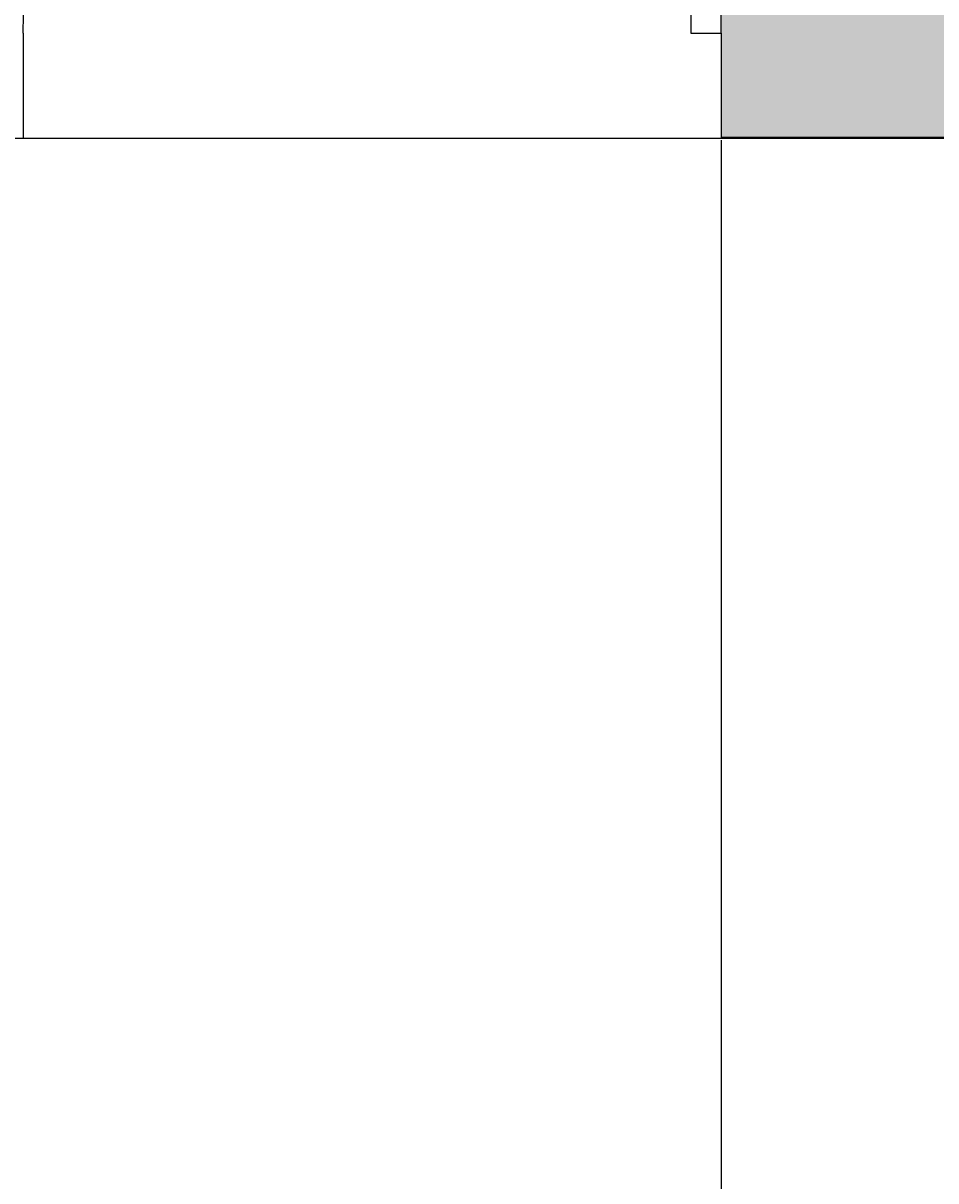
# Model space of a CAD drawing. Units: inches. Extents: x 1998 to 2588, y 1139 to 1977.
# Tile 42 of 134: x 2316 to 2344, y 1557 to 1592. Entities that reach past the tile are written whole.
import ezdxf

# ---------------------------------------------------------------- set-up
doc = ezdxf.new("R2010")
doc.units = ezdxf.units.IN
for name, color, linetype, lineweight in [('A-ANNO-DIMS', 2, 'Continuous', 18), ('A-WALL-PATT', 252, 'Continuous', 13), ('DOOR', 52, 'Continuous', 25), ('WALL', 200, 'Continuous', 35)]:
    doc.layers.add(name, color=color, linetype=linetype, lineweight=lineweight)
doc.styles.get("Standard").update_dxf_attribs({"font": 'arial.ttf'})
doc.dimstyles.get("Standard").update_dxf_attribs({"dimtxt": 0.18, "dimasz": 0.18, "dimexe": 0.18, "dimexo": 0.0625, "dimgap": 0.09, "dimtad": 0, "dimtih": 1, "dimtoh": 1, "dimdec": 4, "dimzin": 0, "dimdsep": 46, "dimtxsty": 'Standard', "dimcen": 0.09, "dimadec": 0, "dimazin": 0, "dimtfac": 1, "dimtdec": 4, "dimtofl": 0, "dimtmove": 0, "dimatfit": 3, "dimfxl": 1, "dimtolj": 1, "dimtzin": 0, "dimarcsym": 0})

# ---------------------------------------------------------------- blocks, each defined once
blk = doc.blocks.new('*U2')
for p, q in [((0, 0), (0, -6)), ((40, 0), (40, -6))]:
    blk.add_line(p, q)
blk.add_lwpolyline([(0, 0), (0, 40), (1.75, 40), (1.75, 0)], close=True)
blk.add_arc((0, 0), 40, 0, 90)
blk = doc.blocks.new('*D34')
at = {"layer": 'A-ANNO-DIMS', "color": 0, "lineweight": -2, "transparency": 16777216}
for p, q in [((2407.91, 1594.732), (1997.843, 1594.732)), ((1998.023, 1594.552), (1998.023, 1558.913)), ((1998.023, 1522.912), (1998.023, 1558.552)), ((2407.91, 1522.732), (1997.843, 1522.732))]:
    blk.add_line(p, q, dxfattribs=at)
at = {"layer": 'A-ANNO-DIMS', "color": 0, "transparency": 16777216}
for points in [[(1997.993, 1594.552), (1998.053, 1594.552), (1998.023, 1594.732)], [(1997.993, 1522.912), (1998.053, 1522.912), (1998.023, 1522.732)]]:
    blk.add_solid(points, dxfattribs=at)
at = {"layer": 'Defpoints', "color": 0, "transparency": 16777216}
for p in [(1998.023, 1594.732), (2407.973, 1594.732), (2407.973, 1522.732)]:
    blk.add_point(p, dxfattribs=at)
at = {"layer": 'A-ANNO-DIMS', "color": 0, "transparency": 16777216, "insert": (1998.023, 1558.732), "char_height": 0.18, "attachment_point": 5}
blk.add_mtext('\\A1;72', dxfattribs=at)
blk = doc.blocks.new('*D42')
at = {"layer": 'A-ANNO-DIMS', "color": 0, "lineweight": -2, "transparency": 16777216}
for p, q in [((2287.535, 1588.732), (2588.309, 1588.732)), ((2588.129, 1588.552), (2588.129, 1555.914)), ((2588.129, 1522.912), (2588.129, 1555.55)), ((2287.535, 1522.732), (2588.309, 1522.732))]:
    blk.add_line(p, q, dxfattribs=at)
at = {"layer": 'A-ANNO-DIMS', "color": 0, "transparency": 16777216}
for points in [[(2588.099, 1588.552), (2588.159, 1588.552), (2588.129, 1588.732)], [(2588.099, 1522.912), (2588.159, 1522.912), (2588.129, 1522.732)]]:
    blk.add_solid(points, dxfattribs=at)
at = {"layer": 'Defpoints', "color": 0, "transparency": 16777216}
for p in [(2287.473, 1588.732), (2588.129, 1588.732), (2287.473, 1522.732)]:
    blk.add_point(p, dxfattribs=at)
at = {"layer": 'A-ANNO-DIMS', "color": 0, "transparency": 16777216, "insert": (2588.129, 1555.732), "char_height": 0.18, "attachment_point": 5}
blk.add_mtext('\\A1;66', dxfattribs=at)
blk = doc.blocks.new('*D44')
at = {"layer": 'A-ANNO-DIMS', "color": 0, "lineweight": -2, "transparency": 16777216}
for p, q in [((2295.414, 1588.67), (2295.414, 1138.602)), ((2337.287, 1588.67), (2337.287, 1138.602)), ((2295.594, 1138.782), (2315.953, 1138.782)), ((2337.107, 1138.782), (2316.748, 1138.782))]:
    blk.add_line(p, q, dxfattribs=at)
at = {"layer": 'A-ANNO-DIMS', "color": 0, "transparency": 16777216}
for points in [[(2295.594, 1138.812), (2295.594, 1138.752), (2295.414, 1138.782)], [(2337.107, 1138.812), (2337.107, 1138.752), (2337.287, 1138.782)]]:
    blk.add_solid(points, dxfattribs=at)
at = {"layer": 'Defpoints', "color": 0, "transparency": 16777216}
for p in [(2295.414, 1588.732), (2337.287, 1588.732), (2337.287, 1138.782)]:
    blk.add_point(p, dxfattribs=at)
at = {"layer": 'A-ANNO-DIMS', "color": 0, "transparency": 16777216, "insert": (2316.35, 1138.782), "char_height": 0.18, "attachment_point": 5}
blk.add_mtext('\\A1;41.87', dxfattribs=at)

msp = doc.modelspace()

# ---------------------------------------------------------------- hatches: boundary and pattern name
at = {"layer": 'A-WALL-PATT'}
h = msp.add_hatch(color=256, dxfattribs=at)
h.dxf.hatch_style = 1
h.paths.add_polyline_path([(2222.9729, 1888.7324), (2099.4125, 1888.7324), (2099.4125, 1879.7324), (2222.9729, 1879.7324)])
h.paths.add_polyline_path([(2096.9729, 1868.3278), (2087.9729, 1868.3278), (2087.9729, 1775.637), (2096.9729, 1775.637)])
h.paths.add_polyline_path([(2227.4729, 1868.3278), (2222.9729, 1868.3278), (2222.9729, 1774.3318), (2227.4729, 1774.3318)])
h.paths.add_polyline_path([(2188.3019, 1759.7324), (2138.6074, 1759.7324), (2099.4125, 1759.7324), (2099.4125, 1755.2324), (2176.9729, 1755.2324), (2188.3019, 1755.2324)])
h.paths.add_polyline_path([(2087.9729, 1759.7324), (2059.4729, 1759.7324), (2059.4729, 1702.7324), (2087.9729, 1702.7324), (2087.9729, 1707.2324), (2063.9729, 1707.2324), (2063.9729, 1755.2324), (2087.9729, 1755.2324)])
h.paths.add_polyline_path([(2096.9729, 1755.2324), (2087.9729, 1755.2324), (2087.9729, 1707.2324), (2096.9729, 1707.2324)])
h.paths.add_polyline_path([(2187.0461, 1707.2324), (2105.9729, 1707.2324), (2096.9729, 1707.2324), (2087.9729, 1707.2324), (2087.9729, 1702.7324), (2105.9729, 1702.7324), (2114.9729, 1702.7324), (2187.0461, 1702.7324)])
h.paths.add_polyline_path([(2181.4729, 1719.2028), (2176.9729, 1719.2028), (2176.9729, 1707.2324), (2181.4729, 1707.2324)])
h.paths.add_polyline_path([(2216.0332, 1588.7324), (2114.9729, 1588.7324), (2105.9729, 1588.7324), (2105.9729, 1584.2324), (2216.0332, 1584.2324)])
h.paths.add_polyline_path([(2077.691, 1588.7324), (2061.4729, 1588.7324), (2061.4729, 1584.2324), (2077.691, 1584.2324)])
h.paths.add_polyline_path([(2105.9729, 1588.7324), (2098.0956, 1588.7324), (2098.0956, 1584.2324), (2105.9729, 1584.2324)])
h.paths.add_polyline_path([(2114.9729, 1596.2642), (2110.1012, 1596.2642), (2105.9729, 1596.2642), (2105.9729, 1588.7324), (2114.9729, 1588.7324)])
h.paths.add_polyline_path([(2114.9729, 1584.2324), (2105.9729, 1584.2324), (2105.9729, 1580.249), (2110.1012, 1580.249), (2114.9729, 1580.249)])
h.paths.add_polyline_path([(2114.9729, 1547.7716), (2110.1012, 1547.7716, -0.0318759), (2105.9729, 1548.035), (2105.9729, 1470.2324), (2108.3775, 1470.2324), (2108.3775, 1465.7324), (2186.2943, 1465.7324), (2186.2943, 1470.2324), (2114.9729, 1470.2324)])
h.paths.add_polyline_path([(2227.4729, 1584.2324), (2222.9729, 1584.2324), (2222.9729, 1486.137), (2227.4729, 1486.137)])
h.paths.add_polyline_path([(2295.4138, 1593.2324), (2227.4729, 1593.2324), (2227.4729, 1588.7324), (2295.4138, 1588.7324), (2295.4138, 1591.8729)])
h.paths.add_polyline_path([(2345.9729, 1627.1165), (2341.4729, 1627.1165), (2341.4729, 1593.2324), (2337.2869, 1593.2324), (2337.2869, 1591.8729), (2337.2869, 1588.7324), (2345.9729, 1588.7324)])
h.paths.add_polyline_path([(2291.9729, 1588.7324), (2287.4729, 1588.7324), (2287.4729, 1522.7324), (2291.9729, 1522.7324)])
h.paths.add_polyline_path([(2291.9729, 1522.7324), (2287.4729, 1522.7324), (2227.4729, 1522.7324), (2227.4729, 1518.2324), (2291.9729, 1518.2324)])
h.paths.add_polyline_path([(2295.7347, 1519.5919), (2295.7347, 1522.7324), (2291.9729, 1522.7324), (2291.9729, 1518.2324), (2295.7347, 1518.2324)])
h.paths.add_polyline_path([(2345.9729, 1522.7324), (2337.6078, 1522.7324), (2337.6078, 1519.5919), (2337.6078, 1518.2324), (2341.4729, 1518.2324), (2341.4729, 1488.5616), (2345.9729, 1488.5616)])
h.paths.add_polyline_path([(2345.9729, 1468.1569), (2341.4729, 1468.1569), (2341.4729, 1374.2324), (2227.4729, 1374.2324), (2227.4729, 1369.7324), (2345.9729, 1369.7324)])
h.paths.add_polyline_path([(2345.9729, 1369.7324), (2341.4729, 1369.7324), (2341.4729, 1362.2324), (2345.9729, 1362.2324)])
h.paths.add_polyline_path([(2345.9729, 1317.7324), (2345.9729, 1322.2324), (2341.4729, 1322.2324), (2341.4729, 1285.137), (2345.9729, 1285.137)], flags=17)
h.paths.add_polyline_path([(2356.2096, 1322.2324), (2345.9729, 1322.2324), (2345.9729, 1317.7324), (2356.2096, 1317.7324), (2356.2096, 1319.3088)], flags=17)
h.paths.add_polyline_path([(2393.9729, 1322.2324), (2375.6999, 1322.2324), (2375.6999, 1319.3088, -0.0202458), (2375.636, 1317.7324), (2393.9729, 1317.7324)], flags=17)
h.paths.add_polyline_path([(2398.4729, 1322.2324), (2393.9729, 1322.2324), (2393.9729, 1317.7324), (2393.9729, 1237.7324), (2345.9729, 1237.7324), (2345.9729, 1264.7324), (2341.4729, 1264.7324), (2341.4729, 1228.7324), (2393.9729, 1228.7324), (2482.7412, 1228.7324), (2482.7412, 1237.7324), (2398.4729, 1237.7324), (2398.4729, 1297.1029)])
h.paths.add_polyline_path([(2398.4729, 1362.2324), (2393.9729, 1362.2324), (2393.9729, 1357.7324), (2398.4729, 1357.7324)])
h.paths.add_polyline_path([(2345.9729, 1329.7549), (2341.4729, 1329.7549), (2341.4729, 1322.2324), (2345.9729, 1322.2324)])

# ---------------------------------------------------------------- linework, layer by layer
at = {"layer": 'WALL'}
msp.add_line((2345.9729, 1588.7324), (2337.2869, 1588.7324), dxfattribs=at)

# ---------------------------------------------------------------- block references
at = {"layer": 'DOOR', "xscale": -0.5234138920659225, "yscale": 0.5234138920659225, "zscale": 0.5234138920659225}
msp.add_blockref('*U2', (2337.2869, 1591.8729), dxfattribs=at)

# ---------------------------------------------------------------- dimensions: what is measured, and where the dimension line sits
at = {"layer": 'A-ANNO-DIMS'}
for base, p1, p2, picture, middle in [((1998.0229, 1594.7324), (2407.9729, 1522.7324), (2407.9729, 1594.7324), '*D34', (1998.0229, 1558.7324)), ((2588.1286, 1588.7324), (2287.4729, 1522.7324), (2287.4729, 1588.7324), '*D42', (2588.1286, 1555.7324))]:
    dim = msp.add_linear_dim(base=base, p1=p1, p2=p2, angle=90, dimstyle='Standard', override={"dimdec": 0, "dimlfac": 1, "dimrnd": 0, "dimzin": 0, "dimdsep": 46, "dimlunit": 2}, dxfattribs=at)
    dim.commit()
    dim.dimension.update_dxf_attribs({"geometry": picture, "text_midpoint": middle})
dim = msp.add_linear_dim(base=(2337.2869, 1138.7824), p1=(2295.4138, 1588.7324), p2=(2337.2869, 1588.7324), dimstyle='Standard', override={"dimdec": 2, "dimlfac": 1, "dimrnd": 0, "dimzin": 0, "dimdsep": 46, "dimlunit": 2}, dxfattribs=at)
dim.commit()
dim.dimension.update_dxf_attribs({"geometry": '*D44', "text_midpoint": (2316.3503, 1138.7824)})

doc.saveas('drawing.dxf')
